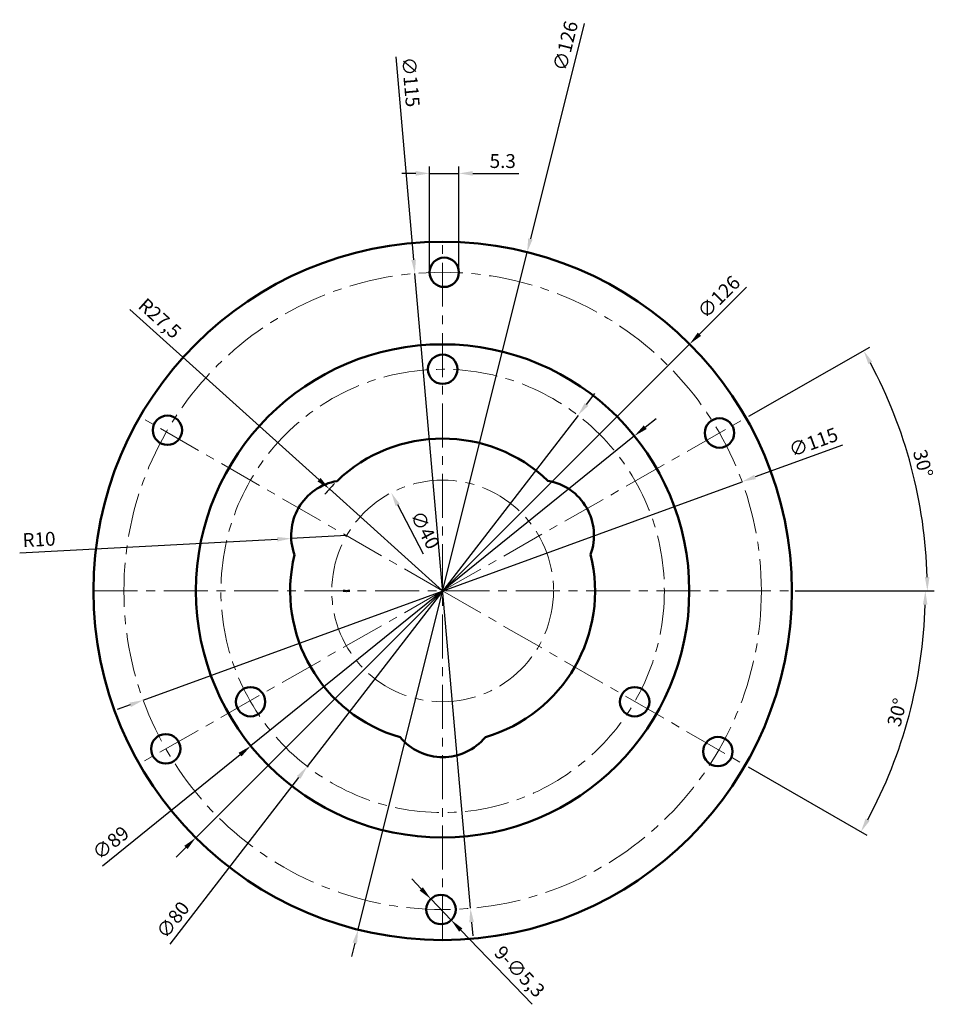
# Model space of a CAD drawing. Units: millimetres. Extents: x 3145 to 3310, y 1466 to 1644.
import ezdxf

# ---------------------------------------------------------------- set-up
doc = ezdxf.new("R2010")
doc.units = ezdxf.units.MM
doc.linetypes.add('CENTER', pattern=[50.8, 31.75, -6.35, 6.35, -6.35])
for name, color, linetype, lineweight in [('M-CNTR', 4, 'CENTER', 18), ('M-DIMS', 2, 'Continuous', 25), ('M-OUTL', 7, 'Continuous', 50)]:
    doc.layers.add(name, color=color, linetype=linetype, lineweight=lineweight)
doc.styles.get("Standard").update_dxf_attribs({"font": 'arial.ttf'})
doc.dimstyles.new('ISO-25', dxfattribs={"dimtxt": 2.5, "dimasz": 2.5, "dimexe": 1.25, "dimexo": 0.625, "dimtad": 1, "dimtxsty": 'Standard', "dimcen": 2.5, "dimadec": 0, "dimazin": 0, "dimtfac": 1, "dimtmove": 0, "dimatfit": 3, "dimfxl": 1, "dimarcsym": 0})

# ---------------------------------------------------------------- blocks, each defined once
blk = doc.blocks.new('*U1')
blk.add_circle((0, 0), 2.65)
blk = doc.blocks.new('*U2')
at = {"layer": 'M-OUTL', "color": 0, "linetype": 'ByBlock', "lineweight": -2, "transparency": 16777216}
for p, rotation in [((3221.84, 1598.1), 60), ((3171.89, 1569.6), 120), ((3171.6, 1512.1), 180), ((3271.2, 1511.6), 300), ((3221.25, 1483.1), 240)]:
    blk.add_blockref('*U1', p, dxfattribs=dict(at, rotation=rotation))
blk.add_blockref('*U1', (3271.49, 1569.1), dxfattribs=at)
blk = doc.blocks.new('*U3')
blk.add_circle((0, 0), 2.65)
blk = doc.blocks.new('*U4')
at = {"layer": 'M-OUTL', "color": 0, "linetype": 'ByBlock', "lineweight": -2, "transparency": 16777216}
blk.add_blockref('*U3', (3221.55, 1580.6), dxfattribs=at)
for p, rotation in [((3186.9, 1520.6), 120), ((3256.19, 1520.6), 240)]:
    blk.add_blockref('*U3', p, dxfattribs=dict(at, rotation=rotation))
blk = doc.blocks.new('*D5')
at = {"layer": 'Defpoints', "color": 0, "transparency": 16777216}
for p in [(3194.23, 1550.06), (3204.21, 1550.58)]:
    blk.add_point(p, dxfattribs=at)
at = {"layer": 'M-DIMS', "color": 0, "lineweight": -2, "transparency": 16777216}
for p, q in [((3145.25, 1547.48), (3191.73, 1549.92)), ((3204.21, 1550.58), (3194.23, 1550.06))]:
    blk.add_line(p, q, dxfattribs=at)
at = {"layer": 'M-DIMS', "color": 0, "transparency": 16777216}
blk.add_solid([(3191.71, 1550.34), (3191.75, 1549.51), (3194.23, 1550.06)], dxfattribs=at)
at = {"layer": 'M-DIMS', "color": 0, "transparency": 16777216, "insert": (3148.75, 1549.57), "char_height": 2.5, "attachment_point": 5, "rotation": 3.0111}
blk.add_mtext('R10', dxfattribs=at)
blk = doc.blocks.new('*D6')
at = {"layer": 'Defpoints', "color": 0, "transparency": 16777216}
for p in [(3201.11, 1559), (3221.55, 1540.6)]:
    blk.add_point(p, dxfattribs=at)
at = {"layer": 'M-DIMS', "color": 0, "lineweight": -2, "transparency": 16777216}
for p, q in [((3165.13, 1591.38), (3199.25, 1560.67)), ((3221.55, 1540.6), (3201.11, 1559))]:
    blk.add_line(p, q, dxfattribs=at)
blk.add_arc((3221.55, 1540.6), 27.5, 135.1459, 140.6162, dxfattribs=at)
at = {"layer": 'M-DIMS', "color": 0, "transparency": 16777216}
blk.add_solid([(3199.53, 1560.98), (3198.97, 1560.36), (3201.11, 1559)], dxfattribs=at)
at = {"layer": 'M-DIMS', "color": 0, "transparency": 16777216, "insert": (3170.32, 1589.56), "char_height": 2.5, "attachment_point": 5, "rotation": 318.0119}
blk.add_mtext('R27,5', dxfattribs=at)
blk = doc.blocks.new('*D7')
at = {"layer": 'Defpoints', "color": 0, "transparency": 16777216}
for p in [(3266.1, 1585.14), (3177, 1496.05)]:
    blk.add_point(p, dxfattribs=at)
at = {"layer": 'M-DIMS', "color": 0, "lineweight": -2, "transparency": 16777216}
for p, q in [((3276.34, 1595.39), (3267.86, 1586.91)), ((3177, 1496.05), (3266.1, 1585.14)), ((3175.23, 1494.29), (3173.46, 1492.52))]:
    blk.add_line(p, q, dxfattribs=at)
at = {"layer": 'M-DIMS', "color": 0, "transparency": 16777216}
for points in [[(3267.57, 1587.21), (3268.16, 1586.62), (3266.1, 1585.14)], [(3174.93, 1494.58), (3175.52, 1493.99), (3177, 1496.05)]]:
    blk.add_solid(points, dxfattribs=at)
at = {"layer": 'M-DIMS', "color": 0, "transparency": 16777216, "insert": (3271.59, 1593.43), "char_height": 2.5, "attachment_point": 5, "rotation": 44.9975}
blk.add_mtext('∅126', dxfattribs=at)
blk = doc.blocks.new('*D8')
at = {"layer": 'Defpoints', "color": 0, "transparency": 16777216}
for p in [(3275.56, 1560.31), (3167.53, 1520.89)]:
    blk.add_point(p, dxfattribs=at)
at = {"layer": 'M-DIMS', "color": 0, "lineweight": -2, "transparency": 16777216}
for p, q in [((3293.69, 1566.92), (3277.91, 1561.16)), ((3167.53, 1520.89), (3275.56, 1560.31)), ((3165.18, 1520.03), (3162.83, 1519.18))]:
    blk.add_line(p, q, dxfattribs=at)
at = {"layer": 'M-DIMS', "color": 0, "transparency": 16777216}
for points in [[(3277.77, 1561.55), (3278.05, 1560.77), (3275.56, 1560.31)], [(3165.04, 1520.43), (3165.32, 1519.64), (3167.53, 1520.89)]]:
    blk.add_solid(points, dxfattribs=at)
at = {"layer": 'M-DIMS', "color": 0, "transparency": 16777216, "insert": (3288.55, 1567.14), "char_height": 2.5, "attachment_point": 5, "rotation": 20.0433}
blk.add_mtext('∅115', dxfattribs=at)
blk = doc.blocks.new('*D9')
at = {"layer": 'Defpoints', "color": 0, "transparency": 16777216}
for p in [(3219.42, 1485.01), (3223.09, 1481.19)]:
    blk.add_point(p, dxfattribs=at)
at = {"layer": 'M-DIMS', "color": 0, "lineweight": -2, "transparency": 16777216}
for p, q in [((3217.69, 1486.81), (3215.96, 1488.62)), ((3219.42, 1485.01), (3223.09, 1481.19)), ((3237.68, 1465.99), (3224.82, 1479.38))]:
    blk.add_line(p, q, dxfattribs=at)
at = {"layer": 'M-DIMS', "color": 0, "transparency": 16777216}
for points in [[(3217.99, 1487.1), (3217.39, 1486.53), (3219.42, 1485.01)], [(3225.12, 1479.67), (3224.52, 1479.1), (3223.09, 1481.19)]]:
    blk.add_solid(points, dxfattribs=at)
at = {"layer": 'M-DIMS', "color": 0, "transparency": 16777216, "insert": (3235.22, 1471.69), "char_height": 2.5, "attachment_point": 5, "rotation": 313.8344}
blk.add_mtext('9-∅5,3', dxfattribs=at)
blk = doc.blocks.new('*D10')
at = {"layer": 'Defpoints', "color": 0, "transparency": 16777216}
for p in [(3256.15, 1568.57), (3186.94, 1512.62)]:
    blk.add_point(p, dxfattribs=at)
at = {"layer": 'M-DIMS', "color": 0, "lineweight": -2, "transparency": 16777216}
for p, q in [((3258.1, 1570.14), (3260.04, 1571.72)), ((3256.15, 1568.57), (3186.94, 1512.62)), ((3160.16, 1490.98), (3184.99, 1511.05))]:
    blk.add_line(p, q, dxfattribs=at)
at = {"layer": 'M-DIMS', "color": 0, "transparency": 16777216}
for points in [[(3257.84, 1570.47), (3258.36, 1569.82), (3256.15, 1568.57)], [(3184.73, 1511.38), (3185.26, 1510.73), (3186.94, 1512.62)]]:
    blk.add_solid(points, dxfattribs=at)
at = {"layer": 'M-DIMS', "color": 0, "transparency": 16777216, "insert": (3161.86, 1494.89), "char_height": 2.5, "attachment_point": 5, "rotation": 38.9494}
blk.add_mtext('∅89', dxfattribs=at)
blk = doc.blocks.new('*D11')
at = {"layer": 'Defpoints', "color": 0, "transparency": 16777216}
for p in [(3245.97, 1572.28), (3197.12, 1508.92)]:
    blk.add_point(p, dxfattribs=at)
at = {"layer": 'M-DIMS', "color": 0, "lineweight": -2, "transparency": 16777216}
for p, q in [((3247.5, 1574.26), (3249.02, 1576.24)), ((3245.97, 1572.28), (3197.12, 1508.92)), ((3172.4, 1476.85), (3195.59, 1506.94))]:
    blk.add_line(p, q, dxfattribs=at)
at = {"layer": 'M-DIMS', "color": 0, "transparency": 16777216}
for points in [[(3247.17, 1574.51), (3247.83, 1574), (3245.97, 1572.28)], [(3195.26, 1507.2), (3195.92, 1506.69), (3197.12, 1508.92)]]:
    blk.add_solid(points, dxfattribs=at)
at = {"layer": 'M-DIMS', "color": 0, "transparency": 16777216, "insert": (3173.14, 1481.04), "char_height": 2.5, "attachment_point": 5, "rotation": 52.3673}
blk.add_mtext('∅80', dxfattribs=at)
blk = doc.blocks.new('*D12')
at = {"layer": 'Defpoints', "color": 0, "transparency": 16777216}
for p in [(3212.28, 1558.32), (3230.81, 1522.88)]:
    blk.add_point(p, dxfattribs=at)
at = {"layer": 'M-DIMS', "color": 0, "lineweight": -2, "transparency": 16777216}
blk.add_line((3218.09, 1547.21), (3213.44, 1556.11), dxfattribs=at)
at = {"layer": 'M-DIMS', "color": 0, "transparency": 16777216}
blk.add_solid([(3213.81, 1556.3), (3213.07, 1555.91), (3212.28, 1558.32)], dxfattribs=at)
at = {"layer": 'M-DIMS', "color": 0, "transparency": 16777216, "insert": (3218.09, 1551.46), "char_height": 2.5, "attachment_point": 5, "rotation": 297.6063}
blk.add_mtext('∅40', dxfattribs=at)
blk = doc.blocks.new('*D13')
at = {"layer": 'Defpoints', "color": 0, "transparency": 16777216}
for p in [(3276.26, 1571.82), (3307.69, 1555.64), (3158.55, 1540.6), (3221.55, 1540.6), (3284.55, 1540.6)]:
    blk.add_point(p, dxfattribs=at)
at = {"layer": 'M-DIMS', "color": 0, "lineweight": -2, "transparency": 16777216}
for p, q in [((3276.81, 1572.13), (3298.59, 1584.56)), ((3285.17, 1540.6), (3310.25, 1540.6))]:
    blk.add_line(p, q, dxfattribs=at)
blk.add_arc((3221.55, 1540.6), 87.45, 1.638, 28.0726, dxfattribs=at)
at = {"layer": 'M-DIMS', "color": 0, "transparency": 16777216}
for points in [[(3298.34, 1581.55), (3299.07, 1581.95), (3297.5, 1583.94)], [(3309.38, 1543.1), (3308.54, 1543.09), (3309, 1540.6)]]:
    blk.add_solid(points, dxfattribs=at)
at = {"layer": 'M-DIMS', "color": 0, "transparency": 16777216, "insert": (3307.91, 1563.51), "char_height": 2.5, "attachment_point": 5, "rotation": 284.8553}
blk.add_mtext('30°', dxfattribs=at)
blk = doc.blocks.new('*D14')
at = {"layer": 'Defpoints', "color": 0, "transparency": 16777216}
for p in [(3158.55, 1540.6), (3221.55, 1540.6), (3284.55, 1540.6), (3303.4, 1510.87), (3276.14, 1509.15)]:
    blk.add_point(p, dxfattribs=at)
at = {"layer": 'M-DIMS', "color": 0, "lineweight": -2, "transparency": 16777216}
for p, q in [((3285.17, 1540.6), (3309.88, 1540.6)), ((3276.68, 1508.84), (3298.09, 1496.51))]:
    blk.add_line(p, q, dxfattribs=at)
blk.add_arc((3221.55, 1540.6), 87.09, 331.7022, 358.3552, dxfattribs=at)
at = {"layer": 'M-DIMS', "color": 0, "transparency": 16777216}
for points in [[(3308.18, 1538.1), (3309.02, 1538.09), (3308.63, 1540.6)], [(3298.59, 1499.11), (3297.86, 1499.52), (3297.01, 1497.13)]]:
    blk.add_solid(points, dxfattribs=at)
at = {"layer": 'M-DIMS', "color": 0, "transparency": 16777216, "insert": (3303.84, 1518.59), "char_height": 2.5, "attachment_point": 5, "rotation": 75.0287}
blk.add_mtext('30°', dxfattribs=at)
blk = doc.blocks.new('*D15')
at = {"layer": 'Defpoints', "color": 0, "transparency": 16777216}
for p in [(3224.49, 1615.95), (3219.19, 1598.1), (3224.49, 1598.1)]:
    blk.add_point(p, dxfattribs=at)
at = {"layer": 'M-DIMS', "color": 0, "lineweight": -2, "transparency": 16777216}
for p, q in [((3219.19, 1598.72), (3219.19, 1617.2)), ((3224.49, 1598.72), (3224.49, 1617.2)), ((3216.69, 1615.95), (3214.19, 1615.95)), ((3219.19, 1615.95), (3224.49, 1615.95)), ((3226.99, 1615.95), (3235.29, 1615.95))]:
    blk.add_line(p, q, dxfattribs=at)
at = {"layer": 'M-DIMS', "color": 0, "transparency": 16777216}
for points in [[(3216.69, 1616.37), (3216.69, 1615.53), (3219.19, 1615.95)], [(3226.99, 1616.37), (3226.99, 1615.53), (3224.49, 1615.95)]]:
    blk.add_solid(points, dxfattribs=at)
at = {"layer": 'M-DIMS', "color": 0, "transparency": 16777216, "insert": (3232.39, 1617.85), "char_height": 2.5, "attachment_point": 5}
blk.add_mtext('5.3', dxfattribs=at)
blk = doc.blocks.new('*D16')
at = {"layer": 'Defpoints', "color": 0, "transparency": 16777216}
for p in [(3236.79, 1601.73), (3206.31, 1479.47)]:
    blk.add_point(p, dxfattribs=at)
at = {"layer": 'M-DIMS', "color": 0, "lineweight": -2, "transparency": 16777216}
for p, q in [((3247.08, 1643.01), (3237.39, 1604.15)), ((3206.31, 1479.47), (3236.79, 1601.73)), ((3205.7, 1477.04), (3205.1, 1474.62))]:
    blk.add_line(p, q, dxfattribs=at)
at = {"layer": 'M-DIMS', "color": 0, "transparency": 16777216}
for points in [[(3236.99, 1604.25), (3237.79, 1604.05), (3236.79, 1601.73)], [(3205.3, 1477.14), (3206.1, 1476.94), (3206.31, 1479.47)]]:
    blk.add_solid(points, dxfattribs=at)
at = {"layer": 'M-DIMS', "color": 0, "transparency": 16777216, "insert": (3244.02, 1638.88), "char_height": 2.5, "attachment_point": 5, "rotation": 76.001}
blk.add_mtext('∅126', dxfattribs=at)
blk = doc.blocks.new('*D17')
at = {"layer": 'Defpoints', "color": 0, "transparency": 16777216}
for p in [(3216.53, 1597.88), (3226.56, 1483.32)]:
    blk.add_point(p, dxfattribs=at)
at = {"layer": 'M-DIMS', "color": 0, "lineweight": -2, "transparency": 16777216}
for p, q in [((3213.11, 1636.99), (3216.31, 1600.37)), ((3226.56, 1483.32), (3216.53, 1597.88)), ((3226.78, 1480.83), (3227, 1478.34))]:
    blk.add_line(p, q, dxfattribs=at)
at = {"layer": 'M-DIMS', "color": 0, "transparency": 16777216}
for points in [[(3216.73, 1600.41), (3215.9, 1600.33), (3216.53, 1597.88)], [(3227.19, 1480.86), (3226.36, 1480.79), (3226.56, 1483.32)]]:
    blk.add_solid(points, dxfattribs=at)
at = {"layer": 'M-DIMS', "color": 0, "transparency": 16777216, "insert": (3215.48, 1632.42), "char_height": 2.5, "attachment_point": 5, "rotation": 275.0038}
blk.add_mtext('∅115', dxfattribs=at)

msp = doc.modelspace()

# ---------------------------------------------------------------- linework, layer by layer
at = {"layer": 'M-CNTR', "ltscale": 0.25, "transparency": 33554534}
for p, q in [((3221.545, 1477.599), (3221.545, 1603.599)), ((3221.545, 1540.599), (3166.954, 1572.044)), ((3221.545, 1540.599), (3276.263, 1571.823)), ((3158.545, 1540.599), (3284.545, 1540.599)), ((3221.545, 1540.599), (3166.827, 1509.375)), ((3221.545, 1540.599), (3276.136, 1509.153))]:
    msp.add_line(p, q, dxfattribs=at)
for radius in [57.5, 40, 20]:
    msp.add_circle((3221.545, 1540.599), radius, dxfattribs=at)
at = {"layer": 'M-OUTL'}
for radius in [63, 44.5]:
    msp.add_circle((3221.545, 1540.599), radius, dxfattribs=at)
for centre, radius, start, end in [((3221.545, 1540.599), 27.5, 46.27099, 133.84373), ((3204.215, 1550.581), 10, 99.8958, 200.21892), ((3238.856, 1550.616), 10, 339.8958, 80.21892), ((3221.545, 1540.599), 27.5, 166.27099, 253.84373), ((3221.545, 1540.599), 27.5, 286.27099, 13.84373), ((3204.215, 1550.581), 10, 266.6249, 273.3751), ((3221.565, 1520.599), 10, 219.8958, 320.21892)]:
    msp.add_arc(centre, radius, start, end, dxfattribs=at)

# ---------------------------------------------------------------- block references
for name in ['*U2', '*U4']:
    msp.add_blockref(name, (0, 0), dxfattribs=at)

# ---------------------------------------------------------------- dimensions: what is measured, and where the dimension line sits
at = {"layer": 'M-DIMS'}
for p1, p2, override, picture, middle in [((3206.305, 1479.47), (3236.785, 1601.727), {"dimdec": 0, "dimlfac": 1, "dimrnd": 0, "dimzin": 0, "dimdsep": 46, "dimlunit": 2}, '*D16', (3245.929, 1638.405)), ((3226.561, 1483.318), (3216.53, 1597.879), {"dimdec": 0, "dimlfac": 1, "dimrnd": 0, "dimzin": 0, "dimdsep": 46, "dimlunit": 2}, '*D17', (3213.521, 1632.248)), ((3245.969, 1572.276), (3197.121, 1508.921), {"dimclrd": 0, "dimclre": 0, "dimclrt": 0}, '*D11', (3174.7, 1479.841)), ((3256.153, 1568.573), (3186.938, 1512.624), {"dimclrd": 0, "dimclre": 0, "dimclrt": 0}, '*D10', (3163.103, 1493.358)), ((3167.528, 1520.892), (3275.563, 1560.306), {"dimclrd": 0, "dimclre": 0, "dimclrt": 0}, '*D8', (3289.224, 1565.29)), ((3230.813, 1522.876), (3212.277, 1558.322), {"dimclrd": 0, "dimclre": 0, "dimclrt": 0}, '*D12', (3216.342, 1550.549))]:
    dim = msp.add_diameter_dim_2p(p1=p1, p2=p2, dimstyle='ISO-25', override=override, dxfattribs=at)
    dim.commit()
    dim.dimension.update_dxf_attribs({"geometry": picture, "text_midpoint": middle, "dimtype": 163})
dim = msp.add_linear_dim(base=(3224.486, 1615.949), p1=(3219.186, 1598.098), p2=(3224.486, 1598.098), dimstyle='ISO-25', override={"dimdec": 1, "dimlfac": 1, "dimrnd": 0, "dimzin": 0, "dimdsep": 46, "dimlunit": 2}, dxfattribs=at)
dim.commit()
dim.dimension.update_dxf_attribs({"geometry": '*D15', "text_midpoint": (3232.387, 1617.851)})
dim = msp.add_diameter_dim_2p(p1=(3176.996, 1496.053), p2=(3266.095, 1585.144), dimstyle='ISO-25', override={"dimclrd": 0, "dimclre": 0, "dimclrt": 0}, dxfattribs=at)
dim.commit()
dim.dimension.update_dxf_attribs({"geometry": '*D7', "text_midpoint": (3271.593, 1593.429)})
for center, mpoint, picture, middle in [((3221.545, 1540.599), (3201.105, 1558.995), '*D6', (3168.902, 1587.979)), ((3204.215, 1550.581), (3194.229, 1550.056), '*D5', (3148.848, 1547.669))]:
    dim = msp.add_radius_dim(center=center, mpoint=mpoint, dimstyle='ISO-25', override={"dimclrd": 0, "dimclre": 0, "dimclrt": 0}, dxfattribs=at)
    dim.commit()
    dim.dimension.update_dxf_attribs({"geometry": picture, "text_midpoint": middle, "dimtype": 164})
for base, line1, picture, middle in [((3307.694, 1555.639), ((3221.545, 1540.599), (3276.263, 1571.823)), '*D13', (3307.913, 1563.507)), ((3303.402, 1510.867), ((3221.545, 1540.599), (3276.136, 1509.153)), '*D14', (3303.841, 1518.592))]:
    dim = msp.add_angular_dim_2l(base=base, line1=line1, line2=((3158.545, 1540.599), (3284.545, 1540.599)), dimstyle='ISO-25', override={"dimclrd": 0, "dimclre": 0, "dimclrt": 0}, dxfattribs=at)
    dim.commit()
    dim.dimension.update_dxf_attribs({"geometry": picture, "text_midpoint": middle})
dim = msp.add_diameter_dim_2p(p1=(3219.42, 1485.011), p2=(3223.09, 1481.188), text='9-<>', dimstyle='ISO-25', override={"dimclrd": 0, "dimclre": 0, "dimclrt": 0}, dxfattribs=at)
dim.commit()
dim.dimension.update_dxf_attribs({"geometry": '*D9', "text_midpoint": (3233.654, 1470.186), "dimtype": 163})

doc.saveas('drawing.dxf')
